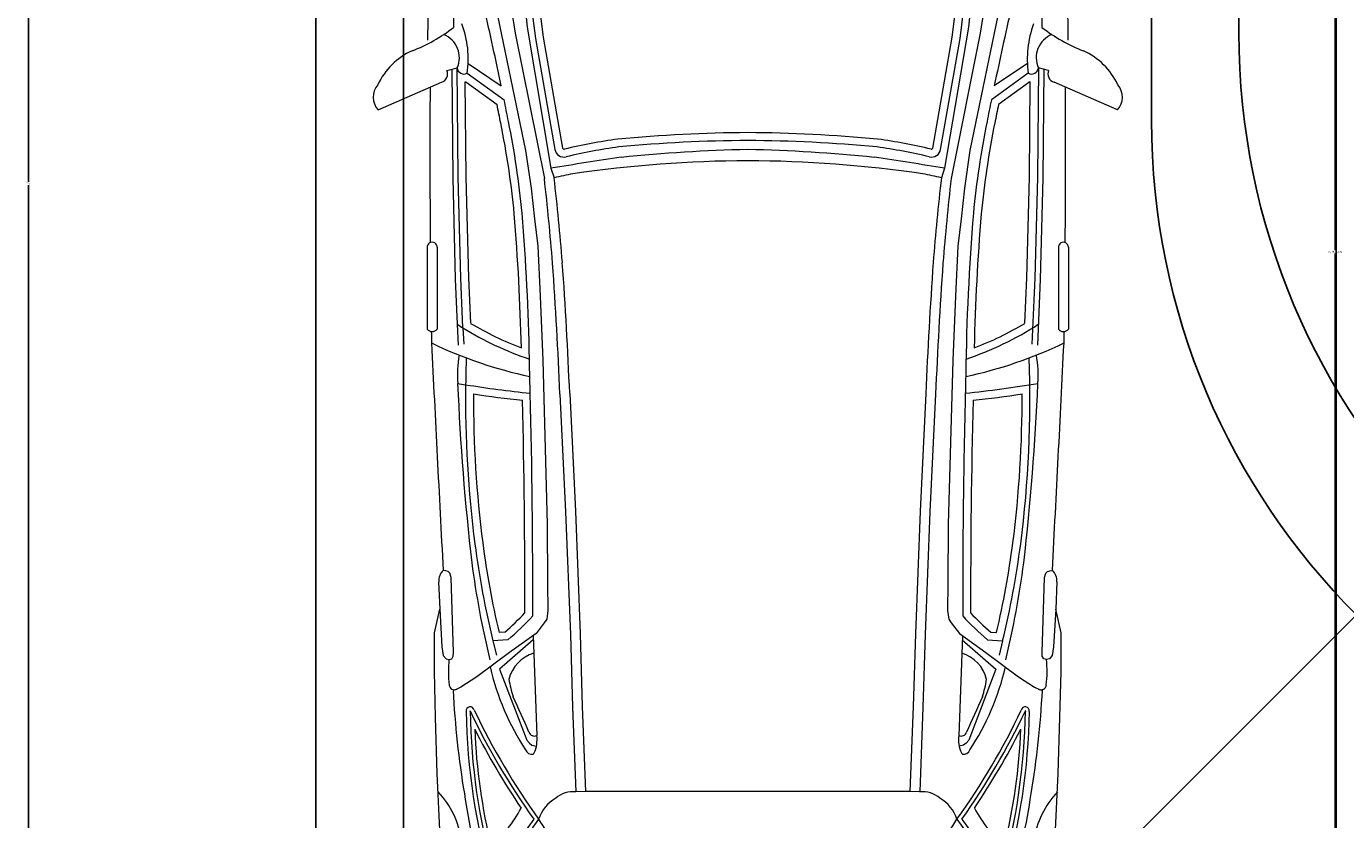
# Model space of a CAD drawing. Units: inches. Extents: x 450 to 1026, y 542 to 1190.
# Tile 2 of 11: x 450 to 586, y 641 to 723. Entities that reach past the tile are written whole.
import ezdxf

# ---------------------------------------------------------------- set-up
doc = ezdxf.new("R2010")
doc.units = ezdxf.units.IN
doc.header["$MEASUREMENT"] = 0
for name, color, linetype, lineweight in [('A-ANNO-DIMS', 2, 'Continuous', 18), ('A-FLOR', 8, 'Continuous', 25), ('C-PROP', 7, 'Continuous', 25), ('C-SITE-VEHC', 8, 'Continuous', 13)]:
    doc.layers.add(name, color=color, linetype=linetype, lineweight=lineweight)
doc.styles.get("Standard").update_dxf_attribs({"font": 'arial.ttf'})
doc.dimstyles.get("Standard").update_dxf_attribs({"dimtxt": 0.18, "dimasz": 0.18, "dimexe": 0.18, "dimexo": 0.0625, "dimgap": 0.09, "dimtad": 0, "dimtih": 1, "dimtoh": 1, "dimdec": 4, "dimzin": 0, "dimdsep": 46, "dimtxsty": 'Standard', "dimcen": 0.09, "dimadec": 0, "dimazin": 0, "dimtfac": 1, "dimtdec": 4, "dimtofl": 0, "dimtmove": 0, "dimatfit": 3, "dimfxl": 1, "dimtolj": 1, "dimtzin": 0, "dimarcsym": 0})

# ---------------------------------------------------------------- blocks, each defined once
blk = doc.blocks.new('A$C27D64469')
for p, q in [((-0.5908, -1.1535), (-0.5454, -1.6151)), ((0.618, -1.1535), (0.5726, -1.6151)), ((-0.563, -1.3311), (-0.5244, -1.6438)), ((-0.5431, -1.3287), (-0.5046, -1.6408)), ((0.5317, -1.6408), (0.5703, -1.3287)), ((0.5515, -1.6438), (0.5901, -1.3311)), ((-0.7946, -1.3764), (-0.7975, -1.6481)), ((-0.7302, -1.3933), (-0.7314, -1.6155)), ((0.7573, -1.3933), (0.7586, -1.6155)), ((0.8217, -1.3764), (0.8246, -1.6481)), ((-0.5904, -1.5351), (-0.5754, -1.6301)), ((0.6175, -1.5351), (0.6026, -1.6301)), ((-0.6294, -1.5396), (-0.5492, -1.9272)), ((0.6565, -1.5396), (0.5764, -1.9272)), ((-0.5754, -1.6301), (-0.5017, -1.9986)), ((-0.5454, -1.6151), (-0.4851, -1.9723)), ((0.5726, -1.6151), (0.5122, -1.9723)), ((0.6026, -1.6301), (0.5289, -1.9986)), ((-0.5244, -1.6438), (-0.475, -1.9247)), ((-0.5046, -1.6408), (-0.4553, -1.9213)), ((0.4824, -1.9213), (0.5317, -1.6408)), ((0.5021, -1.9247), (0.5515, -1.6438)), ((-0.7483, -1.7248), (-0.7225, -1.7182)), ((-0.7364, -1.7217), (-0.7338, -1.998)), ((-0.7199, -1.9952), (-0.7225, -1.7182)), ((-0.6971, -1.7317), (-0.6035, -1.7992)), ((-0.6947, -1.7069), (-0.6109, -1.7637)), ((0.7242, -1.7317), (0.6307, -1.7992)), ((0.7218, -1.7069), (0.638, -1.7637)), ((0.7496, -1.7182), (0.7471, -1.9952)), ((0.7755, -1.7248), (0.7496, -1.7182)), ((0.7635, -1.7217), (0.761, -1.998)), ((-0.9228, -1.8245), (-0.7622, -1.7543)), ((-0.6999, -1.9949), (-0.7021, -1.7537)), ((-0.7009, -1.7536), (-0.6216, -1.8108)), ((0.7281, -1.7536), (0.6487, -1.8108)), ((0.7271, -1.9949), (0.7293, -1.7537)), ((0.9499, -1.8245), (0.7893, -1.7543)), ((-0.5492, -1.9272), (-0.5351, -2.0233)), ((0.5764, -1.9272), (0.5623, -2.0233)), ((-0.7338, -1.998), (-0.7273, -2.254)), ((-0.7134, -2.2512), (-0.7199, -1.9952)), ((-0.6934, -2.2505), (-0.6999, -1.9949)), ((-0.4851, -1.9723), (-0.477, -1.9966)), ((0.5122, -1.9723), (0.5041, -1.9966)), ((0.7206, -2.2505), (0.7271, -1.9949)), ((0.7471, -1.9952), (0.7406, -2.2512)), ((0.761, -1.998), (0.7545, -2.254)), ((-0.5351, -2.0233), (-0.5266, -2.1005)), ((0.5623, -2.0233), (0.5538, -2.1005)), ((-0.5266, -2.1005), (-0.5182, -2.1702)), ((0.5538, -2.1005), (0.5453, -2.1702)), ((-0.5182, -2.1702), (-0.5125, -2.2965)), ((0.5453, -2.1702), (0.5397, -2.2965)), ((-0.7987, -2.1729), (-0.7987, -2.3802)), ((-0.7732, -2.1729), (-0.7732, -2.3802)), ((0.8003, -2.1729), (0.8003, -2.3802)), ((0.8259, -2.1729), (0.8259, -2.3802)), ((-0.7273, -2.254), (-0.7223, -2.368)), ((-0.7078, -2.3771), (-0.7134, -2.2512)), ((-0.6883, -2.3655), (-0.6934, -2.2505)), ((0.7155, -2.3655), (0.7206, -2.2505)), ((0.7406, -2.2512), (0.7332, -2.4181)), ((0.7545, -2.254), (0.7471, -2.4209)), ((-0.5125, -2.2965), (-0.5059, -2.4594)), ((0.5397, -2.2965), (0.5331, -2.4594)), ((-0.7223, -2.368), (-0.7199, -2.4209)), ((-0.7078, -2.3771), (-0.706, -2.4181)), ((-0.5059, -2.4594), (-0.4945, -2.8747)), ((0.5331, -2.4594), (0.5216, -2.8747)), ((-0.4622, -2.5454), (-0.4477, -2.8433)), ((-0.4375, -2.5434), (-0.423, -2.8413)), ((0.4646, -2.5434), (0.4501, -2.8413)), ((0.4894, -2.5454), (0.4748, -2.8433)), ((-0.4477, -2.8433), (-0.4357, -3.1539)), ((-0.423, -2.8413), (-0.4109, -3.152)), ((0.4501, -2.8413), (0.4381, -3.152)), ((0.4748, -2.8433), (0.4628, -3.1539)), ((-0.4945, -2.8747), (-0.4935, -3.0236)), ((0.5216, -2.8747), (0.5207, -3.0236)), ((-0.7516, -2.9924), (-0.758, -2.9914)), ((-0.7456, -2.9946), (-0.7516, -2.9924)), ((-0.7413, -2.9989), (-0.7456, -2.9946)), ((-0.738, -3.0096), (-0.7413, -2.9989)), ((0.7651, -3.0096), (0.7684, -2.9989)), ((0.7684, -2.9989), (0.7727, -2.9946)), ((0.7727, -2.9946), (0.7788, -2.9924)), ((0.7788, -2.9924), (0.7852, -2.9914)), ((-0.7694, -3.0205), (-0.7665, -3.0897)), ((-0.7319, -3.1994), (-0.738, -3.0096)), ((-0.4935, -3.0236), (-0.4926, -3.0933)), ((0.5207, -3.0236), (0.5197, -3.0933)), ((0.759, -3.1994), (0.7651, -3.0096)), ((0.7965, -3.0205), (0.7936, -3.0897)), ((-0.7802, -3.1498), (-0.7665, -3.0897)), ((-0.7665, -3.0897), (-0.761, -3.1849)), ((-0.4926, -3.0933), (-0.4954, -3.115)), ((0.5197, -3.0933), (0.5226, -3.115)), ((0.7936, -3.0897), (0.7882, -3.1849)), ((0.8074, -3.1498), (0.7936, -3.0897)), ((-0.502, -3.1244), (-0.5227, -3.1517)), ((-0.4954, -3.115), (-0.502, -3.1244)), ((0.5226, -3.115), (0.5292, -3.1244)), ((0.5292, -3.1244), (0.5499, -3.1517)), ((-0.7802, -3.248), (-0.7802, -3.1498)), ((-0.594, -3.1673), (-0.632, -3.1701)), ((-0.632, -3.1701), (-0.6229, -3.206)), ((-0.6019, -3.1478), (-0.6165, -3.1489)), ((-0.5298, -3.1676), (-0.615, -3.2421)), ((-0.5227, -3.1517), (-0.5896, -3.1998)), ((-0.5302, -3.1571), (-0.5208, -3.4098)), ((-0.4357, -3.1539), (-0.4303, -3.3385)), ((-0.4109, -3.152), (-0.4055, -3.3366)), ((0.4381, -3.152), (0.4327, -3.3366)), ((0.4628, -3.1539), (0.4574, -3.3385)), ((0.5573, -3.1571), (0.548, -3.4098)), ((0.5499, -3.1517), (0.6167, -3.1998)), ((0.557, -3.1676), (0.6422, -3.2421)), ((0.6212, -3.1673), (0.6592, -3.1701)), ((0.6291, -3.1478), (0.6437, -3.1489)), ((0.6592, -3.1701), (0.65, -3.206)), ((0.8074, -3.248), (0.8074, -3.1498)), ((-0.761, -3.1849), (-0.7577, -3.207)), ((-0.7577, -3.207), (-0.7506, -3.2153)), ((-0.7324, -3.2087), (-0.7319, -3.1994)), ((-0.5896, -3.1998), (-0.6725, -3.261)), ((0.6167, -3.1998), (0.6996, -3.261)), ((0.7595, -3.2087), (0.759, -3.1994)), ((0.7849, -3.207), (0.7778, -3.2153)), ((0.7882, -3.1849), (0.7849, -3.207)), ((-0.7506, -3.2153), (-0.743, -3.2171)), ((-0.743, -3.2171), (-0.7359, -3.2158)), ((-0.7359, -3.2158), (-0.7324, -3.2087)), ((0.7631, -3.2158), (0.7595, -3.2087)), ((0.7702, -3.2171), (0.7631, -3.2158)), ((0.7778, -3.2153), (0.7702, -3.2171)), ((-0.777, -3.3641), (-0.7802, -3.248)), ((-0.6725, -3.261), (-0.713, -3.2874)), ((-0.615, -3.2421), (-0.5463, -3.4221)), ((0.6422, -3.2421), (0.5734, -3.4221)), ((0.6996, -3.261), (0.7401, -3.2874)), ((0.8042, -3.3641), (0.8074, -3.248)), ((-0.7224, -3.2921), (-0.7327, -3.2955)), ((-0.713, -3.2874), (-0.7233, -3.2925)), ((0.7401, -3.2874), (0.7505, -3.2925)), ((0.7495, -3.2921), (0.7599, -3.2955)), ((-0.4303, -3.3385), (-0.4218, -3.5529)), ((-0.4055, -3.3366), (-0.3971, -3.5519)), ((0.4327, -3.3366), (0.4242, -3.5519)), ((0.4574, -3.3385), (0.449, -3.5529)), ((-0.7728, -3.5066), (-0.777, -3.3641)), ((0.8, -3.5066), (0.8042, -3.3641)), ((-0.5463, -3.4221), (-0.5397, -3.4296)), ((-0.5397, -3.4296), (-0.5331, -3.4343)), ((-0.5331, -3.4343), (-0.5217, -3.4366)), ((0.5602, -3.4343), (0.5488, -3.4366)), ((0.5668, -3.4296), (0.5602, -3.4343)), ((0.5734, -3.4221), (0.5668, -3.4296)), ((-0.7654, -3.667), (-0.7728, -3.5066)), ((0.7926, -3.667), (0.8, -3.5066)), ((-0.3971, -3.5519), (-0.4218, -3.5529)), ((0.0136, -3.5519), (-0.3971, -3.5519)), ((0.4242, -3.5519), (0.0136, -3.5519)), ((0.449, -3.5529), (0.4242, -3.5519)), ((-0.5287, -3.6221), (-0.5854, -3.701)), ((-0.5163, -3.6221), (-0.5774, -3.7071)), ((0.5435, -3.6221), (0.6046, -3.7071)), ((0.5559, -3.6221), (0.6126, -3.701))]:
    blk.add_line(p, q)
for centre, radius, start, end in [((-10.825, -3.8887), 10.4328, 11.75206, 12.86028), ((10.8521, -3.8887), 10.4328, 167.13972, 168.24794), ((-0.9818, -1.2945), 0.4071, 290.8732, 307.9458), ((-0.7801, -1.6924), 0.0631, 335.8522, 68.2516), ((-0.9441, -1.6953), 0.2497, 351.6082, 20.7105), ((0.9712, -1.6953), 0.2497, 159.2895, 188.3918), ((0.8072, -1.6924), 0.0631, 111.7484, 204.1478), ((1.0089, -1.2945), 0.4071, 232.0542, 249.1268), ((-0.7607, -1.8385), 0.1804, 114.9135, 154.5523), ((0.7879, -1.8385), 0.1804, 25.4477, 65.0865), ((-0.7685, -1.7333), 0.0219, 286.784, 22.9417), ((-0.7054, -1.7168), 0.0171, 184.6651, 299.1967), ((0.7326, -1.7168), 0.0171, 240.8033, 355.3349), ((0.7957, -1.7333), 0.0219, 157.0583, 253.216), ((-0.8877, -1.7923), 0.0477, 138.9599, 222.5475), ((28.5723, -1.9291), 29.3639, 179.68363, 180.45247), ((-0.7054, -1.7168), 0.0371, 275.0842, 276.9824), ((0.7326, -1.7168), 0.0371, 263.0176, 264.9158), ((-28.5452, -1.9291), 29.3639, 359.54753, 0.31637), ((0.9148, -1.7923), 0.0477, 317.4525, 41.0401), ((-10.825, -3.8887), 10.4328, 11.24656, 11.5533), ((10.8521, -3.8887), 10.4328, 168.4467, 168.75344), ((-10.825, -3.8887), 10.4128, 11.24635, 11.51036), ((10.8521, -3.8887), 10.4128, 168.48964, 168.75365), ((-2.7812, -2.2979), 2.2132, 5.4405, 11.4681), ((-2.7812, -2.2979), 2.2332, 5.4374, 11.4671), ((2.8083, -2.2979), 2.2332, 168.5329, 174.5626), ((2.8083, -2.2979), 2.2132, 168.5319, 174.5595), ((-0.1284, -3.2729), 1.3868, 97.7498, 103.4471), ((0.034, -5.6085), 3.7262, 90.3146, 95.3817), ((0.034, -5.6085), 3.7062, 90.3163, 95.3753), ((-0.0069, -5.6085), 3.7262, 84.6183, 89.6854), ((-0.0069, -5.6085), 3.7062, 84.6247, 89.6837), ((0.1556, -3.2729), 1.3868, 76.5529, 82.2502), ((-0.4518, -1.9207), 0.0236, 189.9743, 283.4471), ((-0.4518, -1.9207), 0.00357, 189.9743, 283.4471), ((-0.1284, -3.2729), 1.3668, 97.7671, 103.4471), ((0.1214, -6.2334), 4.3098, 91.434, 95.7038), ((-0.0943, -6.2334), 4.3098, 84.2962, 88.566), ((0.1556, -3.2729), 1.3668, 76.5529, 82.2329), ((0.4789, -1.9207), 0.0236, 256.5529, 350.0257), ((0.4789, -1.9207), 0.00357, 256.5529, 350.0257), ((2.8455, -23.0231), 21.3127, 98.50598, 98.99062), ((0.0355, -5.2091), 3.2558, 90.3851, 98.2136), ((-0.0083, -5.2091), 3.2558, 81.7864, 89.6149), ((-2.8184, -23.0231), 21.3127, 81.00938, 81.49402), ((-6.4408, -2.6841), 5.9785, 4.51893, 6.58421), ((-0.0958, -3.6836), 1.7295, 101.1311, 102.7329), ((-6.416, -2.6821), 5.9785, 4.51893, 6.58421), ((0.1229, -3.6836), 1.7295, 77.2671, 78.8689), ((6.4432, -2.6821), 5.9785, 173.41579, 175.48107), ((6.4679, -2.6841), 5.9785, 173.41579, 175.48107), ((-6.2705, -2.56), 5.7121, 1.3286, 4.7387), ((-6.2705, -2.56), 5.7321, 1.03863, 4.73991), ((6.2976, -2.56), 5.7321, 175.26009, 179.33379), ((6.2976, -2.56), 5.7121, 175.2613, 178.6714), ((-0.7859, -2.1729), 0.0128, 359.8097, 180.1903), ((0.8131, -2.1729), 0.0128, 359.8097, 180.1903), ((-11.1621, -2.9794), 10.7086, 2.32274, 4.10377), ((-11.1373, -2.9775), 10.7086, 2.32274, 4.10377), ((11.1645, -2.9775), 10.7086, 175.89623, 177.67726), ((11.1892, -2.9794), 10.7086, 175.89623, 177.67726), ((-0.2816, -1.6867), 0.8114, 237.1024, 238.3082), ((-0.2816, -1.6867), 0.7914, 239.0709, 249.4088), ((0.3087, -1.6867), 0.8114, 288.5207, 302.8976), ((0.3087, -1.6867), 0.7914, 290.5912, 300.9291), ((-0.7859, -2.3704), 0.0161, 217.6419, 322.3581), ((28.5723, -1.9291), 29.3639, 180.89229, 180.9487), ((-0.2816, -1.6867), 0.8114, 238.3082, 251.4793), ((0.8131, -2.3704), 0.0161, 217.6419, 322.3581), ((-28.5452, -1.9291), 29.3639, 359.0513, 359.10771), ((145.5619, 4.7984), 146.5271, 182.82189, 183.047472), ((-0.3074, -1.4152), 1.1094, 244.3519, 257.9711), ((0.3345, -1.4152), 1.1094, 282.0289, 295.6481), ((-145.5348, 4.7984), 146.5271, 356.952528, 357.17811), ((-0.4463, -2.4963), 0.2758, 169.4971, 184.519), ((2.1845, -2.5566), 2.8858, 177.9428, 179.2929), ((-6.2705, -2.56), 5.7321, 0.66621, 1.03863), ((-2.1573, -2.5566), 2.8858, 352.6735, 2.0572), ((0.4735, -2.4963), 0.2758, 355.481, 10.5029), ((-21.144, -3.0635), 20.6131, 1.44842, 1.58522), ((21.1711, -3.0635), 20.6131, 178.41478, 180.12035), ((-0.2547, 0.2402), 2.7971, 260.3968, 260.8181), ((5.4584, -2.2589), 6.1852, 182.40058, 186.62429), ((2.1845, -2.5566), 2.8858, 179.2929, 187.3265), ((-0.2547, 0.2402), 2.7971, 260.8181, 264.1988), ((0.2819, 0.2402), 2.7971, 275.8012, 279.6032), ((-5.4313, -2.2589), 6.1852, 353.37571, 357.59942), ((-0.2547, 0.2402), 2.8171, 261.2916, 263.8402), ((2.1845, -2.5566), 2.8658, 179.7551, 187.3262), ((-21.144, -3.0635), 20.5931, 359.90118, 1.39956), ((-21.144, -3.0635), 20.6131, 359.87965, 1.44842), ((21.1711, -3.0635), 20.5931, 178.60044, 180.09882), ((0.2819, 0.2402), 2.8171, 276.1598, 278.7084), ((-2.1573, -2.5566), 2.8658, 352.6738, 0.2449), ((1.5917, -2.6291), 2.2886, 187.4191, 193.6744), ((1.5917, -2.6291), 2.2686, 187.4195, 193.2465), ((-1.5646, -2.6291), 2.2686, 346.7535, 352.5805), ((-1.5646, -2.6291), 2.2886, 346.3256, 352.5809), ((1.584, -2.6769), 2.2886, 187.4191, 193.6744), ((-1.5568, -2.6769), 2.2886, 346.3256, 352.5809), ((-0.7323, -3.0182), 0.0371, 133.8458, 183.4773), ((0.7594, -3.0182), 0.0371, 356.5227, 46.1542), ((-0.9762, -2.7051), 0.5797, 310.2112, 317.1922), ((-0.9762, -2.7051), 0.5997, 309.5861, 317.9444), ((1.0033, -2.7051), 0.5997, 222.0556, 230.4139), ((1.0033, -2.7051), 0.5797, 222.8078, 229.7888), ((-0.5023, -3.2896), 0.0919, 106.6274, 166.1462), ((0.5294, -3.2896), 0.0919, 13.8538, 73.3726), ((-0.4258, -3.2462), 0.3189, 174.7532, 186.4501), ((-0.0025, -3.0882), 0.6536, 193.0984, 213.2489), ((0.0296, -3.0882), 0.6536, 326.7511, 346.9016), ((0.4529, -3.2462), 0.3189, 353.5499, 5.2468), ((-0.2573, -3.2127), 0.3386, 189.3185, 197.018), ((0.2844, -3.2127), 0.3386, 342.982, 350.6815), ((-0.7293, -3.2805), 0.0135, 186.4501, 296.5725), ((1.5487, -3.1796), 2.2844, 182.9075, 189.515), ((-1.5216, -3.1796), 2.2844, 350.485, 357.0925), ((0.7565, -3.2805), 0.0135, 243.4275, 353.5499), ((-0.6895, -3.3475), 0.0103, 9.7306, 189.7306), ((-6.7047, -6.1366), 6.7437, 23.9284, 24.763), ((6.7318, -6.1366), 6.7437, 155.237, 156.0716), ((0.7166, -3.3475), 0.0103, 350.2694, 170.2694), ((0.8768, -3.3275), 1.5766, 180.7904, 196.499), ((-0.6895, -3.3475), 0.000207, 234.3096, 189.7306), ((-0.6997, -3.3492), 0.0101, 0.7904, 9.7306), ((0.9825, -2.5519), 1.8518, 205.4494, 215.3046), ((0.8768, -3.3275), 1.5665, 180.7904, 195.8378), ((0.9825, -2.5519), 1.8417, 205.5332, 215.5287), ((-0.9554, -2.5519), 1.8417, 324.4713, 334.4668), ((-0.9554, -2.5519), 1.8518, 324.6954, 334.5506), ((-0.8496, -3.3275), 1.5665, 344.1622, 359.2096), ((-0.8496, -3.3275), 1.5766, 343.501, 359.2096), ((0.7166, -3.3475), 0.000207, 350.2694, 305.6904), ((0.7268, -3.3492), 0.0101, 170.2694, 179.2096), ((0.8768, -3.3275), 1.5564, 182.4426, 193.5531), ((0.9825, -2.5519), 1.8619, 206.8832, 214.0379), ((-0.5273, -3.3975), 0.0139, 196.0998, 297.49), ((0.5544, -3.3975), 0.0139, 242.51, 343.9002), ((-0.9554, -2.5519), 1.8619, 325.9621, 333.1168), ((-0.8496, -3.3275), 1.5564, 346.4469, 357.5574), ((-0.5991, -3.4208), 0.079, 335.0797, 7.9846), ((0.6263, -3.4208), 0.079, 172.0154, 204.9203), ((-0.5332, -3.4402), 0.0172, 201.6995, 279.6425), ((-0.5326, -3.4521), 0.00559, 294.9923, 338.6694), ((0.5598, -3.4521), 0.00559, 201.3306, 245.0077), ((0.5603, -3.4402), 0.0172, 260.3575, 338.3005), ((-0.931, -3.7054), 0.2213, 7.498, 43.5729), ((0.6722, -3.364), 1.3899, 187.9913, 197.6257), ((-0.421, -3.6549), 0.1008, 121.0416, 161.032), ((-0.4293, -3.6198), 0.0673, 83.5915, 130.4352), ((0.4565, -3.6198), 0.0673, 49.5648, 96.4085), ((0.4482, -3.6549), 0.1008, 18.968, 58.9584), ((-0.645, -3.364), 1.3899, 342.3743, 352.0087), ((0.9581, -3.7054), 0.2213, 136.4271, 172.502), ((-0.9014, -3.4088), 0.388, 313.0938, 331.4872), ((0.9285, -3.4088), 0.388, 208.5128, 226.9062), ((-0.3005, -3.502), 0.247, 209.0915, 245.8956), ((0.3276, -3.502), 0.247, 294.1044, 330.9085)]:
    blk.add_arc(centre, radius, start, end)
blk = doc.blocks.new('*D43')
at = {"layer": 'A-ANNO-DIMS', "color": 0, "lineweight": -2, "transparency": 16777216}
for p, q in [((562.89, 771.86), (584.74, 771.86)), ((584.56, 771.68), (584.56, 699.59)), ((584.56, 627.13), (584.56, 699.22)), ((562.89, 626.95), (584.74, 626.95))]:
    blk.add_line(p, q, dxfattribs=at)
at = {"layer": 'A-ANNO-DIMS', "color": 0, "transparency": 16777216}
for points in [[(584.53, 771.68), (584.59, 771.68), (584.56, 771.86)], [(584.53, 627.13), (584.59, 627.13), (584.56, 626.95)]]:
    blk.add_solid(points, dxfattribs=at)
at = {"layer": 'Defpoints', "color": 0, "transparency": 16777216}
for p in [(562.83, 771.86), (584.56, 771.86), (562.83, 626.95)]:
    blk.add_point(p, dxfattribs=at)
at = {"layer": 'A-ANNO-DIMS', "color": 0, "transparency": 16777216, "insert": (584.56, 699.41), "char_height": 0.18, "attachment_point": 5}
blk.add_mtext('\\A1;VEHICLE 145', dxfattribs=at)
blk = doc.blocks.new('*D53')
at = {"layer": 'A-ANNO-DIMS', "color": 0, "lineweight": -2, "transparency": 16777216}
for p, q in [((479.59, 817.94), (449.87, 817.94)), ((450.05, 817.76), (450.05, 706.62)), ((450.05, 595.12), (450.05, 706.26)), ((797.59, 594.94), (449.87, 594.94))]:
    blk.add_line(p, q, dxfattribs=at)
at = {"layer": 'A-ANNO-DIMS', "color": 0, "transparency": 16777216}
for points in [[(450.02, 817.76), (450.08, 817.76), (450.05, 817.94)], [(450.02, 595.12), (450.08, 595.12), (450.05, 594.94)]]:
    blk.add_solid(points, dxfattribs=at)
at = {"layer": 'Defpoints', "color": 0, "transparency": 16777216}
for p in [(479.65, 817.94), (450.05, 594.94), (797.65, 594.94)]:
    blk.add_point(p, dxfattribs=at)
at = {"layer": 'A-ANNO-DIMS', "color": 0, "transparency": 16777216, "insert": (450.05, 706.44), "char_height": 0.18, "attachment_point": 5}
blk.add_mtext('\\A1;223', dxfattribs=at)
blk = doc.blocks.new('*D56')
at = {"layer": 'A-ANNO-DIMS', "color": 0, "lineweight": -2, "transparency": 16777216}
for p, q in [((488.65, 1150.88), (488.65, 542.16)), ((584.65, 1150.88), (584.65, 542.16)), ((488.83, 542.34), (536.43, 542.34)), ((584.47, 542.34), (536.87, 542.34))]:
    blk.add_line(p, q, dxfattribs=at)
at = {"layer": 'A-ANNO-DIMS', "color": 0, "transparency": 16777216}
for points in [[(488.83, 542.37), (488.83, 542.31), (488.65, 542.34)], [(584.47, 542.37), (584.47, 542.31), (584.65, 542.34)]]:
    blk.add_solid(points, dxfattribs=at)
at = {"layer": 'Defpoints', "color": 0, "transparency": 16777216}
for p in [(488.65, 1150.94), (584.65, 1150.94), (584.65, 542.34)]:
    blk.add_point(p, dxfattribs=at)
at = {"layer": 'A-ANNO-DIMS', "color": 0, "transparency": 16777216, "insert": (536.65, 542.34), "char_height": 0.18, "attachment_point": 5}
blk.add_mtext('\\A1;96', dxfattribs=at)
blk = doc.blocks.new('*D70')
at = {"layer": 'A-ANNO-DIMS', "color": 0, "lineweight": -2, "transparency": 16777216}
for p, q in [((565.65, 713.01), (565.65, 1189.72)), ((565.83, 1189.54), (580.43, 1189.54)), ((595.47, 1189.54), (580.87, 1189.54)), ((595.65, 713.01), (595.65, 1189.72))]:
    blk.add_line(p, q, dxfattribs=at)
at = {"layer": 'A-ANNO-DIMS', "color": 0, "transparency": 16777216}
for points in [[(565.83, 1189.57), (565.83, 1189.51), (565.65, 1189.54)], [(595.47, 1189.57), (595.47, 1189.51), (595.65, 1189.54)]]:
    blk.add_solid(points, dxfattribs=at)
at = {"layer": 'Defpoints', "color": 0, "transparency": 16777216}
for p in [(595.65, 1189.54), (565.65, 712.94), (595.65, 712.94)]:
    blk.add_point(p, dxfattribs=at)
at = {"layer": 'A-ANNO-DIMS', "color": 0, "transparency": 16777216, "insert": (580.65, 1189.54), "char_height": 0.18, "attachment_point": 5}
blk.add_mtext('\\A1;30', dxfattribs=at)
blk = doc.blocks.new('*D75')
at = {"layer": 'A-ANNO-DIMS', "color": 0, "lineweight": -2, "transparency": 16777216}
for p, q in [((637.56, 712.94), (637.74, 712.94)), ((637.65, 712.85), (637.65, 713.03)), ((556.19, 631.48), (586.61, 661.9)), ((556.01, 631.48), (556.19, 631.48))]:
    blk.add_line(p, q, dxfattribs=at)
at = {"layer": 'A-ANNO-DIMS', "color": 0, "transparency": 16777216}
blk.add_solid([(586.59, 661.92), (586.63, 661.88), (586.74, 662.03)], dxfattribs=at)
at = {"layer": 'Defpoints', "color": 0, "transparency": 16777216}
for p in [(637.65, 712.94), (586.74, 662.03)]:
    blk.add_point(p, dxfattribs=at)
at = {"layer": 'A-ANNO-DIMS', "color": 0, "transparency": 16777216, "insert": (555.51, 631.48), "char_height": 0.18, "attachment_point": 5}
blk.add_mtext('\\A1;2X R72', dxfattribs=at)

msp = doc.modelspace()

# ---------------------------------------------------------------- linework, layer by layer
at = {"layer": 'A-FLOR'}
for points in [[(565.6513, 826.9426), (565.6513, 712.9426, 0.41421356), (637.6513, 640.9426), (797.6513, 640.9426)], [(574.6513, 826.9426), (574.6513, 721.9426, 0.41421356), (646.6513, 649.9426), (797.6513, 649.9426)]]:
    msp.add_lwpolyline(points, format="xyb", dxfattribs=at)
at = {"layer": 'C-PROP'}
msp.add_line((479.6513, 1159.9426), (479.6513, 571.9426), dxfattribs=at)

# ---------------------------------------------------------------- block references
at = {"layer": 'C-SITE-VEHC', "xscale": 40.63350989877505, "yscale": 40.63350989877505, "zscale": 40.63350989877505}
msp.add_blockref('A$C27D64469', (523.5448, 788.1608), dxfattribs=at)

# ---------------------------------------------------------------- dimensions: what is measured, and where the dimension line sits
at = {"layer": 'A-ANNO-DIMS'}
for base, p1, p2, picture, middle in [((595.6513, 1189.5426), (565.6513, 712.9426), (595.6513, 712.9426), '*D70', (580.6513, 1189.5426)), ((584.6513, 542.3426), (488.6513, 1150.9426), (584.6513, 1150.9426), '*D56', (536.6513, 542.3426))]:
    dim = msp.add_linear_dim(base=base, p1=p1, p2=p2, dimstyle='Standard', override={"dimdec": 0, "dimlfac": 1, "dimrnd": 0, "dimzin": 0, "dimdsep": 46, "dimlunit": 2}, dxfattribs=at)
    dim.commit()
    dim.dimension.update_dxf_attribs({"geometry": picture, "text_midpoint": middle})
dim = msp.add_linear_dim(base=(450.0513, 594.9426), p1=(479.6513, 817.9426), p2=(797.6513, 594.9426), angle=90, dimstyle='Standard', override={"dimdec": 0, "dimlfac": 1, "dimrnd": 0, "dimzin": 0, "dimdsep": 46, "dimlunit": 2}, dxfattribs=at)
dim.commit()
dim.dimension.update_dxf_attribs({"geometry": '*D53', "text_midpoint": (450.0513, 706.4426)})
dim = msp.add_linear_dim(base=(584.563, 771.8648), p1=(562.8259, 626.9507), p2=(562.8259, 771.8648), angle=90, text='VEHICLE <>', dimstyle='Standard', override={"dimdec": 0, "dimlfac": 1, "dimrnd": 0, "dimzin": 0, "dimdsep": 46, "dimlunit": 2}, dxfattribs=at)
dim.commit()
dim.dimension.update_dxf_attribs({"geometry": '*D43', "text_midpoint": (584.563, 699.4077)})
dim = msp.add_radius_dim(center=(637.6513, 712.9426), mpoint=(586.7403, 662.0303), text='2X <>', dimstyle='Standard', override={"dimdec": 0, "dimlfac": 1, "dimrnd": 0, "dimzin": 0, "dimdsep": 46, "dimlunit": 2}, dxfattribs=at)
dim.commit()
dim.dimension.update_dxf_attribs({"geometry": '*D75', "text_midpoint": (555.5146, 631.4829), "dimtype": 164})

doc.saveas('drawing.dxf')
